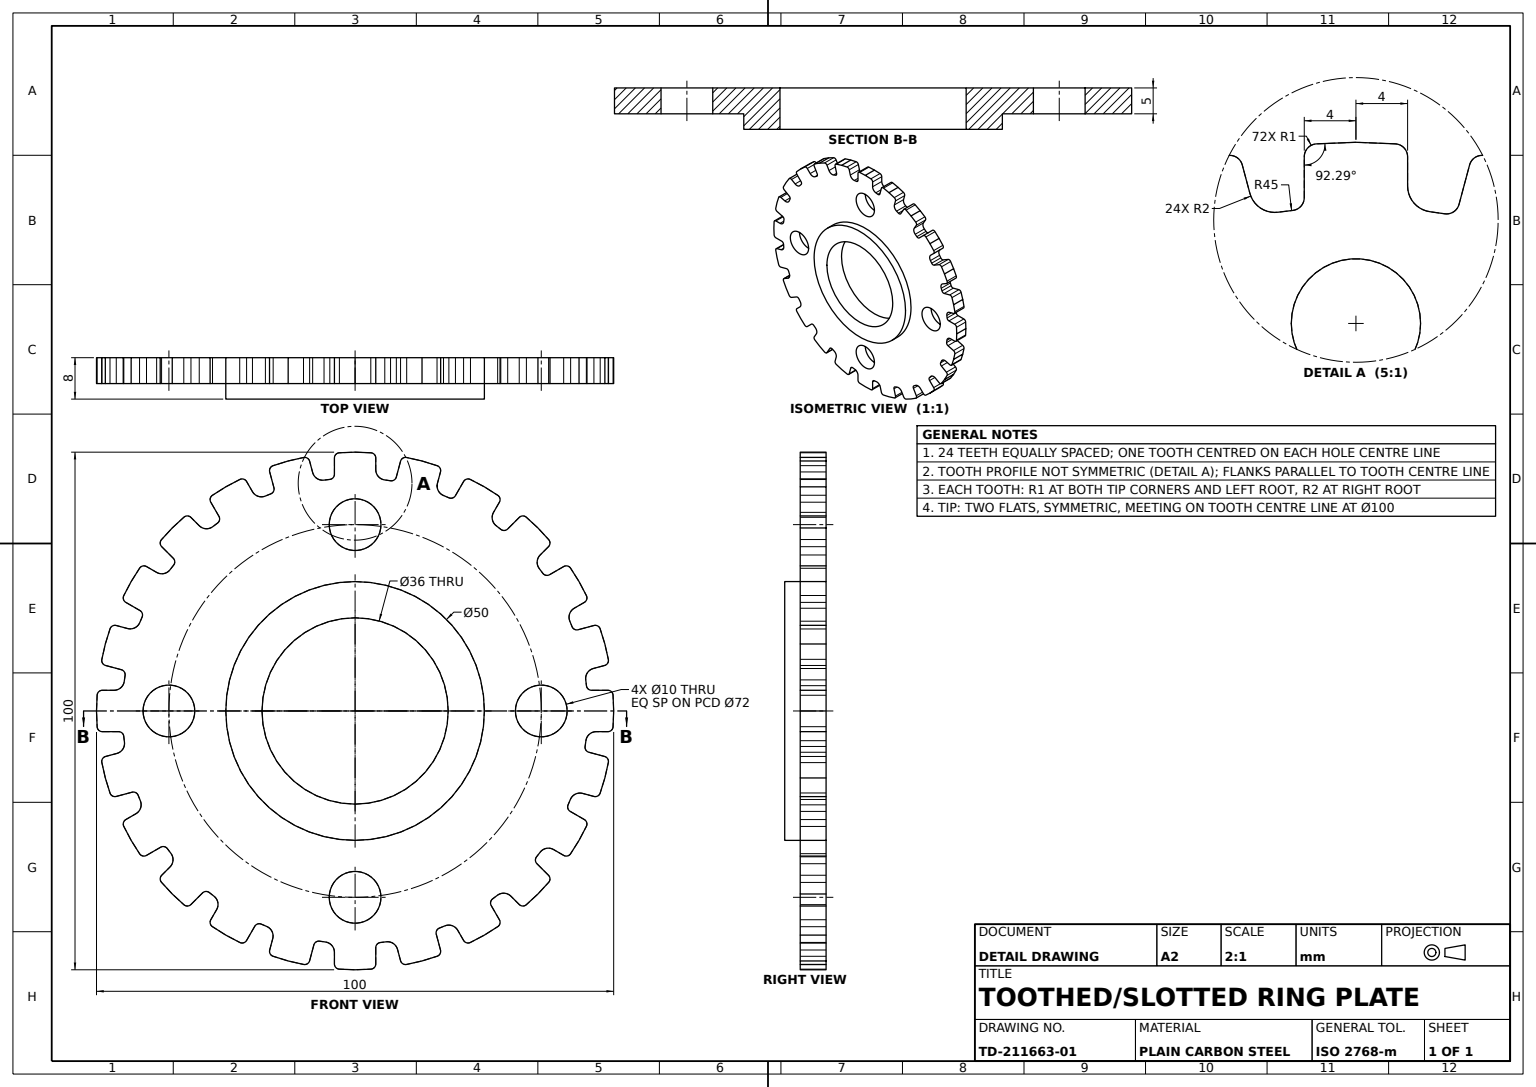
SolidWorks part; units mm, degrees
material "Plain Carbon Steel"
ref_plane "Front Plane" through (0, 0, 0) normal (0, 0, 1) x (1, 0, 0)
ref_plane "Top Plane" through (0, 0, 0) normal (0, 1, 0) x (1, 0, 0)
ref_plane "Right Plane" through (0, 0, 0) normal (1, 0, 0) x (0, 0, -1)
sketch "Toothed Plate Profile Sketch" plane through (0, 0, 0) normal (0, 0, 1) x (1, 0, 0)
  line L0 (0, 0) -> (0, 50) construction
  line L1 (0, 50) -> (-3.0368, 49.8784)
  line L2 (0, 50) -> (3.0368, 49.8784)
  line L3 (3.9968, 48.8792) -> (3.9968, 46.6159)
  line L4 (-3.9968, 48.8792) -> (-3.9968, 45.7278)
  line L5 (8.7903, 48.2482) -> (7.9746, 45.2041)
  line L6 (12.941, 48.2963) -> (9.9762, 48.9648)
  line L7 (12.941, 48.2963) -> (15.8428, 47.3929)
  line L8 (16.5115, 46.1793) -> (15.9257, 43.993)
  line L9 (20.9783, 44.3291) -> (19.4026, 41.5998)
  line L10 (25, 43.3013) -> (22.3093, 44.7144)
  line L11 (25, 43.3013) -> (27.5692, 41.6776)
  line L12 (27.9009, 40.3323) -> (26.7693, 38.3721)
  line L13 (31.7367, 37.389) -> (29.5083, 35.1606)
  line L14 (35.3553, 35.3553) -> (33.122, 37.4167)
  line L15 (35.3553, 35.3553) -> (37.4167, 33.122)
  line L16 (37.389, 31.7367) -> (35.7886, 30.1362)
  line L17 (40.3323, 27.9009) -> (37.603, 26.3252)
  line L18 (43.3013, 25) -> (41.6776, 27.5692)
  line L19 (43.3013, 25) -> (44.7144, 22.3093)
  line L20 (44.3291, 20.9783) -> (42.3689, 19.8466)
  line L21 (46.1793, 16.5115) -> (43.1352, 15.6958)
  line L22 (48.2963, 12.941) -> (47.3929, 15.8428)
  line L23 (48.2963, 12.941) -> (48.9648, 9.9762)
  line L24 (48.2482, 8.7903) -> (46.0619, 8.2045)
  line L25 (48.8792, 3.9968) -> (45.7278, 3.9968)
  line L26 (50, 0) -> (49.8784, 3.0368)
  line L27 (50, 0) -> (49.8784, -3.0368)
  line L28 (48.8792, -3.9968) -> (46.6159, -3.9968)
  line L29 (48.2482, -8.7903) -> (45.2041, -7.9746)
  line L30 (48.2963, -12.941) -> (48.9648, -9.9762)
  line L31 (48.2963, -12.941) -> (47.3929, -15.8428)
  line L32 (46.1793, -16.5115) -> (43.993, -15.9257)
  line L33 (44.3291, -20.9783) -> (41.5998, -19.4026)
  line L34 (43.3013, -25) -> (44.7144, -22.3093)
  line L35 (43.3013, -25) -> (41.6776, -27.5692)
  line L36 (40.3323, -27.9009) -> (38.3721, -26.7693)
  line L37 (37.389, -31.7367) -> (35.1606, -29.5083)
  line L38 (35.3553, -35.3553) -> (37.4167, -33.122)
  line L39 (35.3553, -35.3553) -> (33.122, -37.4167)
  line L40 (31.7367, -37.389) -> (30.1362, -35.7886)
  line L41 (27.9009, -40.3323) -> (26.3252, -37.603)
  line L42 (25, -43.3013) -> (27.5692, -41.6776)
  line L43 (25, -43.3013) -> (22.3093, -44.7144)
  line L44 (20.9783, -44.3291) -> (19.8466, -42.3689)
  line L45 (16.5115, -46.1793) -> (15.6958, -43.1352)
  line L46 (12.941, -48.2963) -> (15.8428, -47.3929)
  line L47 (12.941, -48.2963) -> (9.9762, -48.9648)
  line L48 (8.7903, -48.2482) -> (8.2045, -46.0619)
  line L49 (3.9968, -48.8792) -> (3.9968, -45.7278)
  line L50 (0, -50) -> (3.0368, -49.8784)
  line L51 (0, -50) -> (-3.0368, -49.8784)
  line L52 (-3.9968, -48.8792) -> (-3.9968, -46.6159)
  line L53 (-8.7903, -48.2482) -> (-7.9746, -45.2041)
  line L54 (-12.941, -48.2963) -> (-9.9762, -48.9648)
  line L55 (-12.941, -48.2963) -> (-15.8428, -47.3929)
  line L56 (-16.5115, -46.1793) -> (-15.9257, -43.993)
  line L57 (-20.9783, -44.3291) -> (-19.4026, -41.5998)
  line L58 (-25, -43.3013) -> (-22.3093, -44.7144)
  line L59 (-25, -43.3013) -> (-27.5692, -41.6776)
  line L60 (-27.9009, -40.3323) -> (-26.7693, -38.3721)
  line L61 (-31.7367, -37.389) -> (-29.5083, -35.1606)
  line L62 (-35.3553, -35.3553) -> (-33.122, -37.4167)
  line L63 (-35.3553, -35.3553) -> (-37.4167, -33.122)
  line L64 (-37.389, -31.7367) -> (-35.7886, -30.1362)
  line L65 (-40.3323, -27.9009) -> (-37.603, -26.3252)
  line L66 (-43.3013, -25) -> (-41.6776, -27.5692)
  line L67 (-43.3013, -25) -> (-44.7144, -22.3093)
  line L68 (-44.3291, -20.9783) -> (-42.3689, -19.8466)
  line L69 (-46.1793, -16.5115) -> (-43.1352, -15.6958)
  line L70 (-48.2963, -12.941) -> (-47.3929, -15.8428)
  line L71 (-48.2963, -12.941) -> (-48.9648, -9.9762)
  line L72 (-48.2482, -8.7903) -> (-46.0619, -8.2045)
  line L73 (-48.8792, -3.9968) -> (-45.7278, -3.9968)
  line L74 (-50, 0) -> (-49.8784, -3.0368)
  line L75 (-50, 0) -> (-49.8784, 3.0368)
  line L76 (-48.8792, 3.9968) -> (-46.6159, 3.9968)
  line L77 (-48.2482, 8.7903) -> (-45.2041, 7.9746)
  line L78 (-48.2963, 12.941) -> (-48.9648, 9.9762)
  line L79 (-48.2963, 12.941) -> (-47.3929, 15.8428)
  line L80 (-46.1793, 16.5115) -> (-43.993, 15.9257)
  line L81 (-44.3291, 20.9783) -> (-41.5998, 19.4026)
  line L82 (-43.3013, 25) -> (-44.7144, 22.3093)
  line L83 (-43.3013, 25) -> (-41.6776, 27.5692)
  line L84 (-40.3323, 27.9009) -> (-38.3721, 26.7693)
  line L85 (-37.389, 31.7367) -> (-35.1606, 29.5083)
  line L86 (-35.3553, 35.3553) -> (-37.4167, 33.122)
  line L87 (-35.3553, 35.3553) -> (-33.122, 37.4167)
  line L88 (-31.7367, 37.389) -> (-30.1362, 35.7886)
  line L89 (-27.9009, 40.3323) -> (-26.3252, 37.603)
  line L90 (-25, 43.3013) -> (-27.5692, 41.6776)
  line L91 (-25, 43.3013) -> (-22.3093, 44.7144)
  line L92 (-20.9783, 44.3291) -> (-19.8466, 42.3689)
  line L93 (-16.5115, 46.1793) -> (-15.6958, 43.1352)
  line L94 (-12.941, 48.2963) -> (-15.8428, 47.3929)
  line L95 (-12.941, 48.2963) -> (-9.9762, 48.9648)
  line L96 (-8.7903, 48.2482) -> (-8.2045, 46.0619)
  arc A2 (-4.8882, 44.7337) -> (-6.0057, 44.5974) centre (0, 0) ccw
  arc A3 (-3.0368, 49.8784) -> (-3.9968, 48.8792) centre (-2.9968, 48.8792) ccw
  arc A5 (-4.8882, 44.7337) -> (-3.9968, 45.7278) centre (-4.9968, 45.7278) ccw
  arc A6 (3.9968, 48.8792) -> (3.0368, 49.8784) centre (2.9968, 48.8792) ccw
  arc A8 (3.9968, 46.6159) -> (5.7416, 44.6322) centre (5.9968, 46.6159) ccw
  arc A9 (6.8563, 44.4746) -> (7.9746, 45.2041) centre (7.0087, 45.4629) ccw
  arc A10 (9.9762, 48.9648) -> (8.7903, 48.2482) centre (9.7562, 47.9893) ccw
  arc A11 (16.5115, 46.1793) -> (15.8428, 47.3929) centre (15.5456, 46.4381) ccw
  arc A12 (15.9257, 43.993) -> (17.0976, 41.6254) centre (17.8575, 43.4754) ccw
  arc A13 (18.1336, 41.1846) -> (19.4026, 41.5998) centre (18.5365, 42.0998) ccw
  arc A14 (22.3093, 44.7144) -> (20.9783, 44.3291) centre (21.8443, 43.8291) ccw
  arc A15 (27.9009, 40.3323) -> (27.5692, 41.6776) centre (27.0349, 40.8323) ccw
  arc A16 (26.7693, 38.3721) -> (27.2885, 35.7818) centre (28.5013, 37.3721) ccw
  arc A17 (28.1751, 35.088) -> (29.5083, 35.1606) centre (28.8012, 35.8677) ccw
  arc A18 (33.122, 37.4167) -> (31.7367, 37.389) centre (32.4438, 36.6819) ccw
  arc A19 (37.389, 31.7367) -> (37.4167, 33.122) centre (36.6819, 32.4438) ccw
  arc A20 (35.7886, 30.1362) -> (35.6197, 27.4998) centre (37.2028, 28.722) ccw
  arc A21 (36.2965, 26.6001) -> (37.603, 26.3252) centre (37.103, 27.1913) ccw
  arc A22 (41.6776, 27.5692) -> (40.3323, 27.9009) centre (40.8323, 27.0349) ccw
  arc A23 (44.3291, 20.9783) -> (44.7144, 22.3093) centre (43.8291, 21.8443) ccw
  arc A24 (42.3689, 19.8466) -> (41.5234, 17.3437) centre (43.3689, 18.1145) ccw
  arc A25 (41.9443, 16.2996) -> (43.1352, 15.6958) centre (42.8764, 16.6618) ccw
  arc A26 (47.3929, 15.8428) -> (46.1793, 16.5115) centre (46.4381, 15.5456) ccw
  arc A27 (48.2482, 8.7903) -> (48.9648, 9.9762) centre (47.9893, 9.7562) ccw
  arc A28 (46.0619, 8.2045) -> (44.5974, 6.0057) centre (46.5795, 6.2726) ccw
  arc A29 (44.7337, 4.8882) -> (45.7278, 3.9968) centre (45.7278, 4.9968) ccw
  arc A30 (49.8784, 3.0368) -> (48.8792, 3.9968) centre (48.8792, 2.9968) ccw
  arc A31 (48.8792, -3.9968) -> (49.8784, -3.0368) centre (48.8792, -2.9968) ccw
  arc A32 (46.6159, -3.9968) -> (44.6322, -5.7416) centre (46.6159, -5.9968) ccw
  arc A33 (44.4746, -6.8563) -> (45.2041, -7.9746) centre (45.4629, -7.0087) ccw
  arc A34 (48.9648, -9.9762) -> (48.2482, -8.7903) centre (47.9893, -9.7562) ccw
  arc A35 (46.1793, -16.5115) -> (47.3929, -15.8428) centre (46.4381, -15.5456) ccw
  arc A36 (43.993, -15.9257) -> (41.6254, -17.0976) centre (43.4754, -17.8575) ccw
  arc A37 (41.1846, -18.1336) -> (41.5998, -19.4026) centre (42.0998, -18.5365) ccw
  arc A38 (44.7144, -22.3093) -> (44.3291, -20.9783) centre (43.8291, -21.8443) ccw
  arc A39 (40.3323, -27.9009) -> (41.6776, -27.5692) centre (40.8323, -27.0349) ccw
  arc A40 (38.3721, -26.7693) -> (35.7818, -27.2885) centre (37.3721, -28.5013) ccw
  arc A41 (35.088, -28.1751) -> (35.1606, -29.5083) centre (35.8677, -28.8012) ccw
  arc A42 (37.4167, -33.122) -> (37.389, -31.7367) centre (36.6819, -32.4438) ccw
  arc A43 (31.7367, -37.389) -> (33.122, -37.4167) centre (32.4438, -36.6819) ccw
  arc A44 (30.1362, -35.7886) -> (27.4998, -35.6197) centre (28.722, -37.2028) ccw
  arc A45 (26.6001, -36.2965) -> (26.3252, -37.603) centre (27.1913, -37.103) ccw
  arc A46 (27.5692, -41.6776) -> (27.9009, -40.3323) centre (27.0349, -40.8323) ccw
  arc A47 (20.9783, -44.3291) -> (22.3093, -44.7144) centre (21.8443, -43.8291) ccw
  arc A48 (19.8466, -42.3689) -> (17.3437, -41.5234) centre (18.1145, -43.3689) ccw
  arc A49 (16.2996, -41.9443) -> (15.6958, -43.1352) centre (16.6618, -42.8764) ccw
  arc A50 (15.8428, -47.3929) -> (16.5115, -46.1793) centre (15.5456, -46.4381) ccw
  arc A51 (8.7903, -48.2482) -> (9.9762, -48.9648) centre (9.7562, -47.9893) ccw
  arc A52 (8.2045, -46.0619) -> (6.0057, -44.5974) centre (6.2726, -46.5795) ccw
  arc A53 (4.8882, -44.7337) -> (3.9968, -45.7278) centre (4.9968, -45.7278) ccw
  arc A54 (3.0368, -49.8784) -> (3.9968, -48.8792) centre (2.9968, -48.8792) ccw
  arc A55 (-3.9968, -48.8792) -> (-3.0368, -49.8784) centre (-2.9968, -48.8792) ccw
  arc A56 (-3.9968, -46.6159) -> (-5.7416, -44.6322) centre (-5.9968, -46.6159) ccw
  arc A57 (-6.8563, -44.4746) -> (-7.9746, -45.2041) centre (-7.0087, -45.4629) ccw
  arc A58 (-9.9762, -48.9648) -> (-8.7903, -48.2482) centre (-9.7562, -47.9893) ccw
  arc A59 (-16.5115, -46.1793) -> (-15.8428, -47.3929) centre (-15.5456, -46.4381) ccw
  arc A60 (-15.9257, -43.993) -> (-17.0976, -41.6254) centre (-17.8575, -43.4754) ccw
  arc A61 (-18.1336, -41.1846) -> (-19.4026, -41.5998) centre (-18.5365, -42.0998) ccw
  arc A62 (-22.3093, -44.7144) -> (-20.9783, -44.3291) centre (-21.8443, -43.8291) ccw
  arc A63 (-27.9009, -40.3323) -> (-27.5692, -41.6776) centre (-27.0349, -40.8323) ccw
  arc A64 (-26.7693, -38.3721) -> (-27.2885, -35.7818) centre (-28.5013, -37.3721) ccw
  arc A65 (-28.1751, -35.088) -> (-29.5083, -35.1606) centre (-28.8012, -35.8677) ccw
  arc A66 (-33.122, -37.4167) -> (-31.7367, -37.389) centre (-32.4438, -36.6819) ccw
  arc A67 (-37.389, -31.7367) -> (-37.4167, -33.122) centre (-36.6819, -32.4438) ccw
  arc A68 (-35.7886, -30.1362) -> (-35.6197, -27.4998) centre (-37.2028, -28.722) ccw
  arc A69 (-36.2965, -26.6001) -> (-37.603, -26.3252) centre (-37.103, -27.1913) ccw
  arc A70 (-41.6776, -27.5692) -> (-40.3323, -27.9009) centre (-40.8323, -27.0349) ccw
  arc A71 (-44.3291, -20.9783) -> (-44.7144, -22.3093) centre (-43.8291, -21.8443) ccw
  arc A72 (-42.3689, -19.8466) -> (-41.5234, -17.3437) centre (-43.3689, -18.1145) ccw
  arc A73 (-41.9443, -16.2996) -> (-43.1352, -15.6958) centre (-42.8764, -16.6618) ccw
  arc A74 (-47.3929, -15.8428) -> (-46.1793, -16.5115) centre (-46.4381, -15.5456) ccw
  arc A75 (-48.2482, -8.7903) -> (-48.9648, -9.9762) centre (-47.9893, -9.7562) ccw
  arc A76 (-46.0619, -8.2045) -> (-44.5974, -6.0057) centre (-46.5795, -6.2726) ccw
  arc A77 (-44.7337, -4.8882) -> (-45.7278, -3.9968) centre (-45.7278, -4.9968) ccw
  arc A78 (-49.8784, -3.0368) -> (-48.8792, -3.9968) centre (-48.8792, -2.9968) ccw
  arc A79 (-48.8792, 3.9968) -> (-49.8784, 3.0368) centre (-48.8792, 2.9968) ccw
  arc A80 (-46.6159, 3.9968) -> (-44.6322, 5.7416) centre (-46.6159, 5.9968) ccw
  arc A81 (-44.4746, 6.8563) -> (-45.2041, 7.9746) centre (-45.4629, 7.0087) ccw
  arc A82 (-48.9648, 9.9762) -> (-48.2482, 8.7903) centre (-47.9893, 9.7562) ccw
  arc A83 (-46.1793, 16.5115) -> (-47.3929, 15.8428) centre (-46.4381, 15.5456) ccw
  arc A84 (-43.993, 15.9257) -> (-41.6254, 17.0976) centre (-43.4754, 17.8575) ccw
  arc A85 (-41.1846, 18.1336) -> (-41.5998, 19.4026) centre (-42.0998, 18.5365) ccw
  arc A86 (-44.7144, 22.3093) -> (-44.3291, 20.9783) centre (-43.8291, 21.8443) ccw
  arc A87 (-40.3323, 27.9009) -> (-41.6776, 27.5692) centre (-40.8323, 27.0349) ccw
  arc A88 (-38.3721, 26.7693) -> (-35.7818, 27.2885) centre (-37.3721, 28.5013) ccw
  arc A89 (-35.088, 28.1751) -> (-35.1606, 29.5083) centre (-35.8677, 28.8012) ccw
  arc A90 (-37.4167, 33.122) -> (-37.389, 31.7367) centre (-36.6819, 32.4438) ccw
  arc A91 (-31.7367, 37.389) -> (-33.122, 37.4167) centre (-32.4438, 36.6819) ccw
  arc A92 (-30.1362, 35.7886) -> (-27.4998, 35.6197) centre (-28.722, 37.2028) ccw
  arc A93 (-26.6001, 36.2965) -> (-26.3252, 37.603) centre (-27.1913, 37.103) ccw
  arc A94 (-27.5692, 41.6776) -> (-27.9009, 40.3323) centre (-27.0349, 40.8323) ccw
  arc A95 (-20.9783, 44.3291) -> (-22.3093, 44.7144) centre (-21.8443, 43.8291) ccw
  arc A96 (-19.8466, 42.3689) -> (-17.3437, 41.5234) centre (-18.1145, 43.3689) ccw
  arc A97 (-16.2996, 41.9443) -> (-15.6958, 43.1352) centre (-16.6618, 42.8764) ccw
  arc A98 (-15.8428, 47.3929) -> (-16.5115, 46.1793) centre (-15.5456, 46.4381) ccw
  arc A99 (-8.7903, 48.2482) -> (-9.9762, 48.9648) centre (-9.7562, 47.9893) ccw
  arc A100 (-8.2045, 46.0619) -> (-6.0057, 44.5974) centre (-6.2726, 46.5795) ccw
  arc A102 (-16.2996, 41.9443) -> (-17.3437, 41.5234) centre (0, 0) ccw
  arc A103 (-26.6001, 36.2965) -> (-27.4998, 35.6197) centre (0, 0) ccw
  arc A104 (-35.088, 28.1751) -> (-35.7818, 27.2885) centre (0, 0) ccw
  arc A105 (-41.1846, 18.1336) -> (-41.6254, 17.0976) centre (0, 0) ccw
  arc A106 (-44.4746, 6.8563) -> (-44.6322, 5.7416) centre (0, 0) ccw
  arc A107 (-44.7337, -4.8882) -> (-44.5974, -6.0057) centre (0, 0) ccw
  arc A108 (-41.9443, -16.2996) -> (-41.5234, -17.3437) centre (0, 0) ccw
  arc A109 (-36.2965, -26.6001) -> (-35.6197, -27.4998) centre (0, 0) ccw
  arc A110 (-28.1751, -35.088) -> (-27.2885, -35.7818) centre (0, 0) ccw
  arc A111 (-18.1336, -41.1846) -> (-17.0976, -41.6254) centre (0, 0) ccw
  arc A112 (-6.8563, -44.4746) -> (-5.7416, -44.6322) centre (0, 0) ccw
  arc A113 (4.8882, -44.7337) -> (6.0057, -44.5974) centre (0, 0) ccw
  arc A114 (16.2996, -41.9443) -> (17.3437, -41.5234) centre (0, 0) ccw
  arc A115 (26.6001, -36.2965) -> (27.4998, -35.6197) centre (0, 0) ccw
  arc A116 (35.088, -28.1751) -> (35.7818, -27.2885) centre (0, 0) ccw
  arc A117 (41.1846, -18.1336) -> (41.6254, -17.0976) centre (0, 0) ccw
  arc A118 (44.4746, -6.8563) -> (44.6322, -5.7416) centre (0, 0) ccw
  arc A119 (44.7337, 4.8882) -> (44.5974, 6.0057) centre (0, 0) ccw
  arc A120 (41.9443, 16.2996) -> (41.5234, 17.3437) centre (0, 0) ccw
  arc A121 (36.2965, 26.6001) -> (35.6197, 27.4998) centre (0, 0) ccw
  arc A122 (28.1751, 35.088) -> (27.2885, 35.7818) centre (0, 0) ccw
  arc A123 (18.1336, 41.1846) -> (17.0976, 41.6254) centre (0, 0) ccw
  arc A124 (6.8563, 44.4746) -> (5.7416, 44.6322) centre (0, 0) ccw
  dimension "D1" = 6.0736
  dimension "D2" = 90
  dimension "D3" = 2
  dimension "D4" = 2
  dimension "D6" = 2
  dimension "D7" = 4
  dimension "D5" = 3.9968
  dimension "D8" = 24
  dimension "D9" = 2.2634
extrude "Toothed Flange Plate 24T" add sketch "Toothed Plate Profile Sketch" along normal blind 5
sketch "Hub Ring Sketch" plane through (0, 0, 5) normal (0, 0, 1) x (1, 0, 0)
  circle A0 centre (0, 0) radius 18
  circle A1 centre (0, 0) radius 25
  dimension "D1" = 36
  dimension "D2" = 50
extrude "Hub Ring Ø50" add sketch "Hub Ring Sketch" along normal blind 3
sketch "Centre Bore Sketch" plane through (0, 0, 5) normal (0, 0, 1) x (1, 0, 0)
  circle A0 centre (0, 0) radius 18
  dimension "D1" = 36
extrude "Centre Bore" cut sketch "Centre Bore Sketch" against normal through all
sketch "Bolt Hole Sketch" plane through (0, 0, 5) normal (0, 0, 1) x (1, 0, 0)
  line L0 (-3.9968, 48.8792) -> (-3.9968, 45.7278) construction
  circle A0 centre (0, 36) radius 5
  dimension "D1" = 10
  dimension "D2" = 36
  dimension "D3" = 3.9968
extrude "Bolt Hole Ø10" cut sketch "Bolt Hole Sketch" against normal through all
pattern_circular "Bolt Hole and Hub Pattern 4x" count 4 over 360 about axis through (0, 0, 0) along (0, 0, 1) of "Bolt Hole Ø10"
